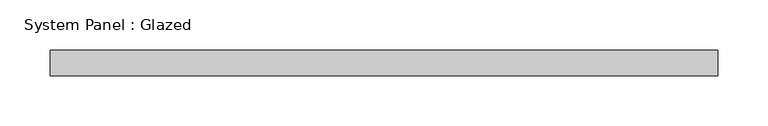
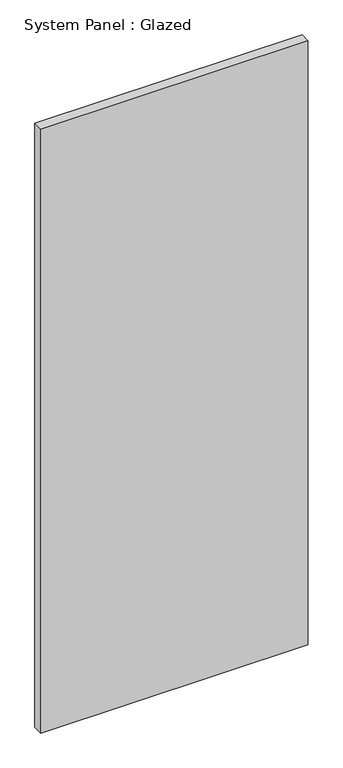
"""IFC4 building model written with IfcOpenShell, lengths in millimetres: plate geometry, System Panel : Glazed."""

from ifc_helpers import new_model, si_unit, origin, origin_with_axes, place, context, project, spatial, polyline, outline, extrude, source, transform, mapped, element, save


def system_panel_glazed_ba9a01dc(model_context):
    return source(origin(), model_context, "Body", "SweptSolid", [
        extrude(outline(polyline([(333.375, 19.05), (-333.375, 19.05), (-333.375, 44.45), (333.375, 44.45), (333.375, 19.05)])), origin_with_axes(), (0.0, 0.0, 1.0), 1592.9882445),
    ])


if __name__ == "__main__":
    model = new_model("IFC4")
    model_context = context("Model", 3, world=origin())
    ifc_project = project(units=[si_unit("LENGTHUNIT", "METRE", prefix="MILLI")], contexts=[model_context])
    site = spatial("IfcSite", under=ifc_project)
    building = spatial("IfcBuilding", under=site)
    placement = place(None, origin())
    system_panel_glazed_shape = system_panel_glazed_ba9a01dc(model_context)
    element("IfcPlate", 1, ObjectType="System Panel : Glazed", at=placement, inside=building, context=model_context, shape_type="MappedRepresentation", body=[
        mapped(system_panel_glazed_shape, transform((0.0, 0.0, 0.0), x_axis=(1.0, 0.0, 0.0), y_axis=(0.0, 1.0, 0.0), z_axis=(0.0, 0.0, 1.0))),
    ])
    save(model, "model.ifc")

# Revit data of these elements
# Type "System Panel : Glazed"
#   Construction Type Id = "GSP4R"
#   Analytic Construction = "1/8 in Pilkington single glazing"
#   Visual Light Transmittance = 0.9
#   Solar Heat Gain Coefficient = 0.86
#   Heat Transfer Coefficient (U) = 1.18115 BTU/(h·ft²·°F)
#   Define Thermal Properties by = 1
# Element 1 (IfcPlate, "System Panel : Glazed")
#   Materials on its faces: "Glass"
# Materials
#   "Glass": class "Glass", colour RGB 0 128 192, transparency 0.75, Description = "Soda Lime Glass", Cost = 0
